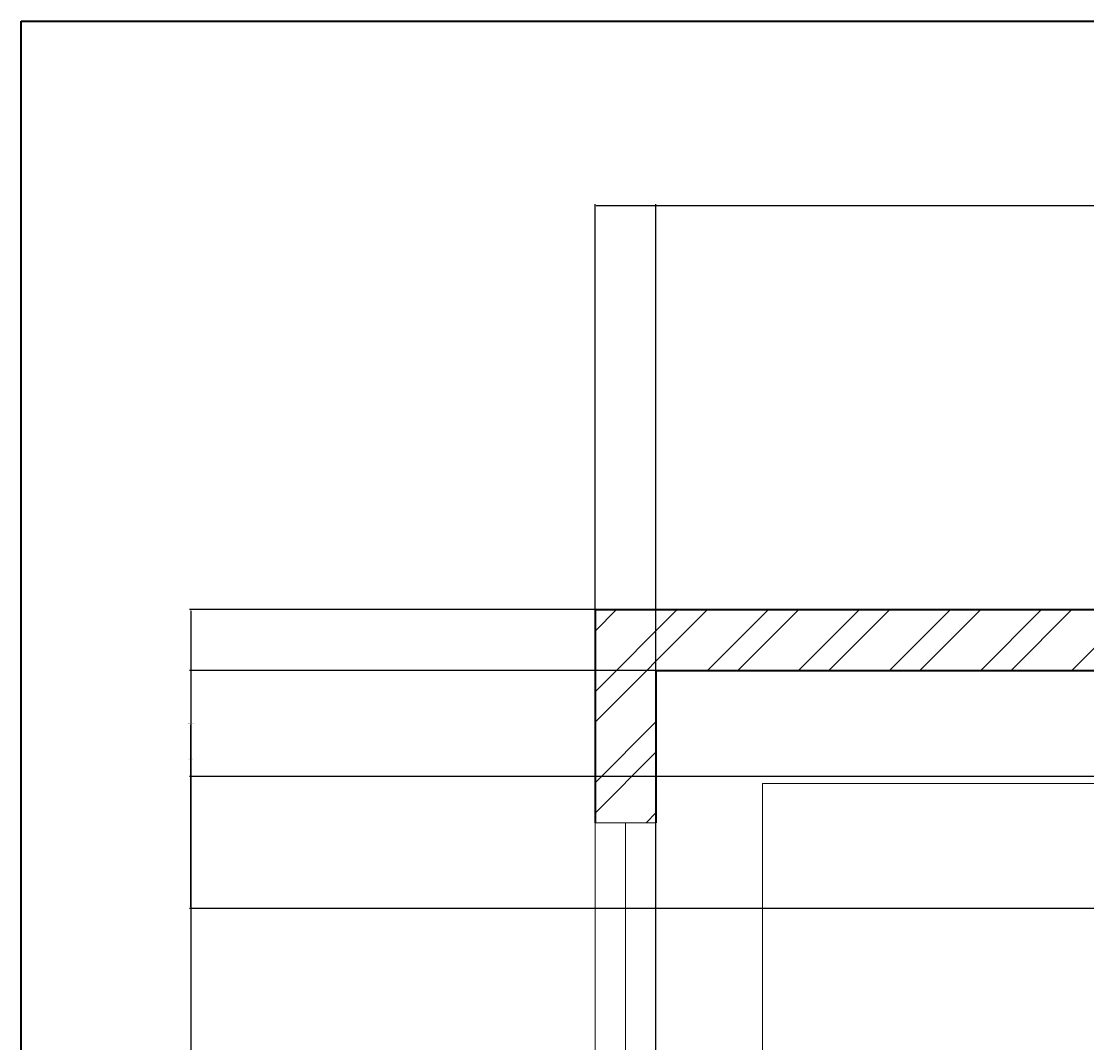
# Model space of a CAD drawing. Units: inches. Extents: x 2552 to 3217, y 1417 to 2737.
# Tile 17 of 25: x 2552 to 2710, y 2585 to 2737. Entities that reach past the tile are written whole.
import ezdxf

# ---------------------------------------------------------------- set-up
doc = ezdxf.new("R2010")
doc.units = ezdxf.units.IN
for name, color, linetype, lineweight in [('A-ANNO-DIMS', 2, 'Continuous', 18), ('A-ANNO-TTLB', 7, 'Continuous', 35), ('A-FLOR-CASE', 9, 'Continuous', 18), ('A-GLAZ', 161, 'Continuous', 18), ('A-WALL', 7, 'Continuous', 35), ('A-WALL-PATT', 217, 'Continuous', 13)]:
    doc.layers.add(name, color=color, linetype=linetype, lineweight=lineweight)
doc.styles.get("Standard").update_dxf_attribs({"font": 'arial.ttf'})
doc.dimstyles.get("Standard").update_dxf_attribs({"dimtxt": 0.18, "dimasz": 0.18, "dimexe": 0.18, "dimexo": 0.0625, "dimgap": 0.09, "dimtad": 0, "dimtih": 1, "dimtoh": 1, "dimdec": 4, "dimzin": 0, "dimdsep": 46, "dimtxsty": 'Standard', "dimcen": 0.09, "dimadec": 0, "dimazin": 0, "dimtfac": 1, "dimtdec": 4, "dimtofl": 0, "dimtmove": 0, "dimatfit": 3, "dimfxl": 1, "dimtolj": 1, "dimtzin": 0, "dimarcsym": 0})

# ---------------------------------------------------------------- blocks, each defined once
blk = doc.blocks.new('WIN-36')
for p, q in [((4.5, 36), (0, 36)), ((0, 36), (9, 36)), ((0, 36), (0, 0)), ((4.5, 0), (4.5, 36)), ((9, 36), (9, 0)), ((0, 0), (9, 0)), ((9, 0), (4.5, 0))]:
    blk.add_line(p, q)
blk = doc.blocks.new('*D50')
at = {"layer": 'A-ANNO-DIMS', "color": 0, "lineweight": -2, "transparency": 16777216}
for p, q in [((2637.29, 2649.51), (2577.37, 2649.51)), ((2577.55, 2649.33), (2577.55, 2096.19)), ((2577.55, 1542.69), (2577.55, 2095.83)), ((2637.29, 1542.51), (2577.37, 1542.51))]:
    blk.add_line(p, q, dxfattribs=at)
at = {"layer": 'A-ANNO-DIMS', "color": 0, "transparency": 16777216}
for points in [[(2577.52, 2649.33), (2577.58, 2649.33), (2577.55, 2649.51)], [(2577.52, 1542.69), (2577.58, 1542.69), (2577.55, 1542.51)]]:
    blk.add_solid(points, dxfattribs=at)
at = {"layer": 'Defpoints', "color": 0, "transparency": 16777216}
for p in [(2577.55, 2649.51), (2637.35, 2649.51), (2637.35, 1542.51)]:
    blk.add_point(p, dxfattribs=at)
at = {"layer": 'A-ANNO-DIMS', "color": 0, "transparency": 16777216, "insert": (2577.55, 2096.01), "char_height": 0.18, "attachment_point": 5}
blk.add_mtext('\\A1;1107', dxfattribs=at)
blk = doc.blocks.new('*D51')
at = {"layer": 'A-ANNO-DIMS', "color": 0, "lineweight": -2, "transparency": 16777216}
for p, q in [((2637.35, 2649.58), (2637.35, 2709.49)), ((2637.53, 2709.31), (2742.71, 2709.31)), ((2848.67, 2709.31), (2743.5, 2709.31)), ((2848.85, 2649.58), (2848.85, 2709.49))]:
    blk.add_line(p, q, dxfattribs=at)
at = {"layer": 'A-ANNO-DIMS', "color": 0, "transparency": 16777216}
for points in [[(2637.53, 2709.34), (2637.53, 2709.28), (2637.35, 2709.31)], [(2848.67, 2709.34), (2848.67, 2709.28), (2848.85, 2709.31)]]:
    blk.add_solid(points, dxfattribs=at)
at = {"layer": 'Defpoints', "color": 0, "transparency": 16777216}
for p in [(2848.85, 2709.31), (2637.35, 2649.51), (2848.85, 2649.51)]:
    blk.add_point(p, dxfattribs=at)
at = {"layer": 'A-ANNO-DIMS', "color": 0, "transparency": 16777216, "insert": (2743.1, 2709.31), "char_height": 0.18, "attachment_point": 5}
blk.add_mtext('\\A1;211.5', dxfattribs=at)
blk = doc.blocks.new('*D64')
at = {"layer": 'A-ANNO-DIMS', "color": 0, "lineweight": -2, "transparency": 16777216}
for p, q in [((2646.35, 1551.58), (2646.35, 2709.49)), ((2646.53, 2709.31), (2802.77, 2709.31)), ((2959.93, 2709.31), (2803.69, 2709.31)), ((2960.11, 1551.58), (2960.11, 2709.49))]:
    blk.add_line(p, q, dxfattribs=at)
at = {"layer": 'A-ANNO-DIMS', "color": 0, "transparency": 16777216}
for points in [[(2646.53, 2709.34), (2646.53, 2709.28), (2646.35, 2709.31)], [(2959.93, 2709.34), (2959.93, 2709.28), (2960.11, 2709.31)]]:
    blk.add_solid(points, dxfattribs=at)
at = {"layer": 'Defpoints', "color": 0, "transparency": 16777216}
for p in [(2960.11, 2709.31), (2646.35, 1551.51), (2960.11, 1551.51)]:
    blk.add_point(p, dxfattribs=at)
at = {"layer": 'A-ANNO-DIMS', "color": 0, "transparency": 16777216, "insert": (2803.23, 2709.31), "char_height": 0.18, "attachment_point": 5}
blk.add_mtext('\\A1;313.76', dxfattribs=at)
blk = doc.blocks.new('*D65')
at = {"layer": 'A-ANNO-DIMS', "color": 0, "lineweight": -2, "transparency": 16777216}
for p, q in [((2908.79, 2649.51), (2577.37, 2649.51)), ((2577.55, 2649.33), (2577.55, 2627.57)), ((2577.55, 2605.46), (2577.55, 2627.21)), ((2908.79, 2605.28), (2577.37, 2605.28))]:
    blk.add_line(p, q, dxfattribs=at)
at = {"layer": 'A-ANNO-DIMS', "color": 0, "transparency": 16777216}
for points in [[(2577.52, 2649.33), (2577.58, 2649.33), (2577.55, 2649.51)], [(2577.52, 2605.46), (2577.58, 2605.46), (2577.55, 2605.28)]]:
    blk.add_solid(points, dxfattribs=at)
at = {"layer": 'Defpoints', "color": 0, "transparency": 16777216}
for p in [(2577.55, 2649.51), (2908.85, 2649.51), (2908.85, 2605.28)]:
    blk.add_point(p, dxfattribs=at)
at = {"layer": 'A-ANNO-DIMS', "color": 0, "transparency": 16777216, "insert": (2577.55, 2627.39), "char_height": 0.18, "attachment_point": 5}
blk.add_mtext('\\A1;44.24', dxfattribs=at)
blk = doc.blocks.new('*D68')
at = {"layer": 'A-ANNO-DIMS', "color": 0, "lineweight": -2, "transparency": 16777216}
for p, q in [((2995.79, 2640.51), (2577.37, 2640.51)), ((2577.55, 2640.33), (2577.55, 2632.84)), ((2577.55, 2624.97), (2577.55, 2632.47)), ((2995.79, 2624.79), (2577.37, 2624.79))]:
    blk.add_line(p, q, dxfattribs=at)
at = {"layer": 'A-ANNO-DIMS', "color": 0, "transparency": 16777216}
for points in [[(2577.52, 2640.33), (2577.58, 2640.33), (2577.55, 2640.51)], [(2577.52, 2624.97), (2577.58, 2624.97), (2577.55, 2624.79)]]:
    blk.add_solid(points, dxfattribs=at)
at = {"layer": 'Defpoints', "color": 0, "transparency": 16777216}
for p in [(2995.85, 2640.51), (2577.55, 2624.79), (2995.85, 2624.79)]:
    blk.add_point(p, dxfattribs=at)
at = {"layer": 'A-ANNO-DIMS', "color": 0, "transparency": 16777216, "insert": (2577.55, 2632.65), "char_height": 0.18, "attachment_point": 5}
blk.add_mtext('\\A1;15.718', dxfattribs=at)

msp = doc.modelspace()

# ---------------------------------------------------------------- hatches: boundary and pattern name
at = {"layer": 'A-WALL-PATT'}
h = msp.add_hatch(dxfattribs=at)
h.set_pattern_fill('ANSI32', color=256)
h.paths.add_polyline_path([(2756.676, 2649.5125), (2637.3535, 2649.5125), (2637.3535, 2617.9626), (2641.8535, 2617.9626), (2646.3535, 2617.9626), (2646.3535, 2640.5125), (2724.3535, 2640.5125), (2724.3535, 2520.5125), (2720.299, 2520.5125), (2720.299, 2516.0125), (2733.4075, 2516.0125), (2733.4075, 2518.2213), (2733.4075, 2520.5125), (2728.8535, 2520.5125), (2728.8535, 2640.5125), (2756.676, 2640.5125)])
h.paths.add_polyline_path([(2848.8535, 2649.5125), (2804.676, 2649.5125), (2804.676, 2640.5125), (2839.8535, 2640.5125), (2839.8535, 2598.3517), (2848.8535, 2598.3517)])
h.paths.add_polyline_path([(2646.3535, 2516.0125), (2697.9593, 2516.0125), (2697.9593, 2518.2625), (2697.9593, 2520.5125), (2646.3535, 2520.5125), (2646.3535, 2581.9626), (2637.3535, 2581.9626), (2637.3535, 2364.3298), (2646.3535, 2364.3298), (2646.3535, 2387.0125), (2724.3535, 2387.0125), (2724.3535, 2267.0125), (2721.0443, 2267.0125), (2721.0443, 2262.5125), (2733.7854, 2262.5125), (2733.7854, 2264.7625), (2733.7854, 2267.0125), (2728.8535, 2267.0125), (2728.8535, 2387.0125), (2839.8535, 2387.0125), (2839.8535, 2363.8387), (2848.8535, 2363.8387), (2848.8535, 2403.7415), (2844.3535, 2403.7415), (2839.8535, 2403.7415), (2839.8535, 2396.0125), (2646.3535, 2396.0125)])
h.paths.add_polyline_path([(2848.8535, 2550.3517), (2844.3535, 2550.3517), (2839.8535, 2550.3517), (2839.8535, 2520.5125), (2801.9195, 2520.5125), (2801.9195, 2518.2625), (2801.9195, 2516.0125), (2839.8535, 2516.0125), (2839.8535, 2507.5813), (2848.8535, 2507.5813)], flags=17)
h.paths.add_polyline_path([(2848.8535, 2483.5813), (2844.3535, 2483.5813), (2839.8535, 2483.5813), (2839.8535, 2468.0125), (2773.8535, 2468.0125), (2773.8535, 2516.0125), (2778.1336, 2516.0125), (2778.1336, 2520.5125), (2766.696, 2520.5125), (2766.696, 2518.2625), (2766.696, 2516.0125), (2769.3535, 2516.0125), (2769.3535, 2463.5125), (2839.8535, 2463.5125), (2839.8535, 2431.0782), (2848.8535, 2431.0782)], flags=17)
h.paths.add_polyline_path([(2917.8535, 2569.2764), (2913.3535, 2569.2764), (2908.8535, 2569.2764), (2908.8535, 2433.001), (2917.8535, 2433.001), (2917.8535, 2516.0125), (2967.486, 2516.0125), (2967.486, 2520.5125), (2917.8535, 2520.5125)])
h.paths.add_polyline_path([(3000.3535, 2640.5125), (2995.8535, 2640.5125), (2995.8535, 2520.5125), (2990.688, 2520.5125), (2990.688, 2516.0125), (3004.0844, 2516.0125), (3004.0844, 2518.2625), (3004.0844, 2520.5125), (3000.3535, 2520.5125)])
h.paths.add_polyline_path([(3120.3535, 2561.3689), (3115.8535, 2561.3689), (3111.3535, 2561.3689), (3111.3535, 2520.5125), (3070.9814, 2520.5125), (3070.9814, 2518.2625), (3070.9814, 2516.0125), (3111.3535, 2516.0125), (3111.3535, 2505.1841), (3120.3535, 2505.1841)])
h.paths.add_polyline_path([(3120.3535, 2481.1841), (3115.8535, 2481.1841), (3111.3535, 2481.1841), (3111.3535, 2468.0125), (3045.3535, 2468.0125), (3045.3535, 2516.0125), (3048.9787, 2516.0125), (3048.9787, 2520.5125), (3036.3395, 2520.5125), (3036.3395, 2516.0125), (3040.8535, 2516.0125), (3040.8535, 2463.5125), (3111.3535, 2463.5125), (3111.3535, 2396.0125), (2917.8535, 2396.0125), (2917.8535, 2403.4124), (2913.3535, 2403.4124), (2908.8535, 2403.4124), (2908.8535, 2182.5756), (2917.8535, 2182.5756), (2917.8535, 2262.5125), (2968.001, 2262.5125), (2968.001, 2264.7625), (2968.001, 2267.0125), (2917.8535, 2267.0125), (2917.8535, 2387.0125), (3111.3535, 2387.0125), (3111.3535, 2352.2435), (3120.3535, 2352.2435)])
h.paths.add_polyline_path([(3120.3535, 2304.2435), (3115.8535, 2304.2435), (3111.3535, 2304.2435), (3111.3535, 2267.0125), (3073.8616, 2267.0125), (3073.8616, 2264.7625), (3073.8616, 2262.5125), (3111.3535, 2262.5125), (3111.3535, 2252.376), (3120.3535, 2252.376)], flags=17)
h.paths.add_polyline_path([(3120.3535, 2228.376), (3115.8535, 2228.376), (3111.3535, 2228.376), (3111.3535, 2214.5125), (3045.3535, 2214.5125), (3045.3535, 2262.5125), (3049.3096, 2262.5125), (3049.3096, 2267.0125), (3035.0125, 2267.0125), (3035.0125, 2262.5125), (3040.8535, 2262.5125), (3040.8535, 2210.0125), (3111.3535, 2210.0125), (3111.3535, 2142.5125), (2917.8535, 2142.5125), (2917.8535, 2150.2408), (2913.3535, 2150.2408), (2908.8535, 2150.2408), (2908.8535, 1924.9905), (2917.8535, 1924.9905), (2917.8535, 2009.0125), (2971.959, 2009.0125), (2971.959, 2011.2625), (2971.959, 2013.5125), (2917.8535, 2013.5125), (2917.8535, 2133.5125), (2995.8535, 2133.5125), (2995.8535, 2013.5125), (2992.1797, 2013.5125), (2992.1797, 2009.0125), (3004.3344, 2009.0125), (3004.3344, 2011.2625), (3004.3344, 2013.5125), (3000.3535, 2013.5125), (3000.3535, 2133.5125), (3111.3535, 2133.5125), (3111.3535, 2115.0291), (3120.3535, 2115.0291)])
h.paths.add_polyline_path([(3000.3535, 2387.0125), (2995.8535, 2387.0125), (2995.8535, 2267.0125), (2991.3326, 2267.0125), (2991.3326, 2262.5125), (3004.1044, 2262.5125), (3004.1044, 2264.7625), (3004.1044, 2267.0125), (3000.3535, 2267.0125)], flags=17)
h.paths.add_polyline_path([(3120.3535, 1973.2388), (3115.8535, 1973.2388), (3111.3535, 1973.2388), (3111.3535, 1961.0125), (3045.3535, 1961.0125), (3045.3535, 2009.0125), (3048.9101, 2009.0125), (3048.9101, 2013.5125), (3037.105, 2013.5125), (3037.105, 2011.2625), (3037.105, 2009.0125), (3040.8535, 2009.0125), (3040.8535, 1956.5125), (3111.3535, 1956.5125), (3111.3535, 1889.0125), (2917.8535, 1889.0125), (2917.8535, 1895.7215), (2913.3535, 1895.7215), (2908.8535, 1895.7215), (2908.8535, 1844.2217), (2917.8535, 1844.2217), (2917.8535, 1880.0125), (3111.3535, 1880.0125), (3111.3535, 1846.9541), (3120.3535, 1846.9541)])
h.paths.add_polyline_path([(3120.3535, 2067.0291), (3111.3535, 2067.0291), (3111.3535, 2013.5125), (3071.3001, 2013.5125), (3071.3001, 2009.0125), (3111.3535, 2009.0125), (3111.3535, 1997.2388), (3120.3535, 1997.2388)], flags=0)
h.paths.add_polyline_path([(3120.3535, 1798.9541), (3115.8535, 1798.9541), (3111.3535, 1798.9541), (3111.3535, 1760.0125), (3071.2497, 1760.0125), (3071.2497, 1757.7625), (3071.2497, 1755.5125), (3111.3535, 1755.5125), (3111.3535, 1746.162), (3120.3535, 1746.2478)])
h.paths.add_polyline_path([(3120.3535, 1722.2049), (3111.3535, 1722.2049), (3111.3535, 1707.5125), (3045.3535, 1707.5125), (3045.3535, 1755.5125), (3048.6624, 1755.5125), (3048.6624, 1760.0125), (3035.3703, 1760.0125), (3035.3703, 1755.5125), (3040.8535, 1755.5125), (3040.8535, 1703.0125), (3111.3535, 1703.0125), (3111.3535, 1635.5125), (2917.8535, 1635.5125), (2917.8535, 1643.1366), (2913.3535, 1643.1366), (2908.8535, 1643.1366), (2908.8535, 1626.5125), (3120.3535, 1626.5125)])
h.paths.add_polyline_path([(2917.8535, 1755.5125), (2973.2287, 1755.5125), (2973.2287, 1757.7625), (2973.2287, 1760.0125), (2917.8535, 1760.0125), (2917.8535, 1808.2217), (2913.3535, 1808.2217), (2908.8535, 1808.2217), (2908.8535, 1676.1665), (2917.8535, 1676.1665)])
h.paths.add_polyline_path([(3000.3535, 1880.0125), (2995.8535, 1880.0125), (2995.8535, 1760.0125), (2992.9329, 1760.0125), (2992.9329, 1755.5125), (3003.8766, 1755.5125), (3003.8766, 1757.7625), (3003.8766, 1760.0125), (3000.3535, 1760.0125)])
h.paths.add_polyline_path([(2848.8535, 1896.6971), (2844.3535, 1896.6971), (2839.8535, 1896.6971), (2839.8535, 1889.0125), (2646.3535, 1889.0125), (2646.3535, 2009.0125), (2700.5253, 2009.0125), (2700.5253, 2011.2625), (2700.5253, 2013.5125), (2646.3535, 2013.5125), (2646.3535, 2053.1812), (2641.8535, 2053.1812), (2637.3535, 2053.1812), (2637.3535, 1836.254), (2646.3535, 1836.254), (2646.3535, 1880.0125), (2724.3535, 1880.0125), (2724.3535, 1760.0125), (2721.2473, 1760.0125), (2721.2473, 1755.5125), (2731.9187, 1755.5125), (2731.9187, 1757.7625), (2731.9187, 1760.0125), (2728.8535, 1760.0125), (2728.8535, 1880.0125), (2839.8535, 1880.0125), (2839.8535, 1840.3813), (2848.8535, 1840.3813)])
h.paths.add_polyline_path([(2848.8535, 1792.3813), (2844.3535, 1792.3813), (2839.8535, 1792.3813), (2839.8535, 1760.0125), (2797.8845, 1760.0125), (2797.8845, 1755.5125), (2839.8535, 1755.5125), (2839.8535, 1743.3688), (2844.3535, 1743.3688), (2848.8535, 1743.3688)], flags=0)
h.paths.add_polyline_path([(2848.8535, 1719.3688), (2844.3535, 1719.3688), (2839.8535, 1719.3688), (2839.8535, 1707.5125), (2773.8535, 1707.5125), (2773.8535, 1755.5125), (2777.716, 1755.5125), (2777.716, 1760.0125), (2760.9247, 1760.0125), (2760.9247, 1757.9721), (2760.9247, 1755.5125), (2769.3535, 1755.5125), (2769.3535, 1703.0125), (2839.8535, 1703.0125), (2839.8535, 1673.0277), (2848.8535, 1672.9407)], flags=0)
h.paths.add_polyline_path([(2646.3535, 1755.5125), (2702.9171, 1755.5125), (2702.9171, 1757.7625), (2702.9171, 1760.0125), (2646.3535, 1760.0125), (2646.3535, 1800.254), (2641.8535, 1800.254), (2637.3535, 1800.254), (2637.3535, 1626.5125), (2848.8535, 1626.5125), (2848.8535, 1643.1187), (2844.3535, 1643.1187), (2839.8535, 1643.1187), (2839.8535, 1635.5125), (2646.3535, 1635.5125)])
h.paths.add_polyline_path([(2848.8535, 2148.8427), (2844.3535, 2148.8427), (2839.8535, 2148.8427), (2839.8535, 2142.5125), (2646.3535, 2142.5125), (2646.3535, 2262.5125), (2701.3562, 2262.5125), (2701.3562, 2264.7625), (2701.3562, 2267.0125), (2646.3535, 2267.0125), (2646.3535, 2328.3298), (2637.3535, 2328.3298), (2637.3535, 2089.1812), (2646.3535, 2089.1812), (2646.3535, 2133.5125), (2839.8535, 2133.5125), (2839.8535, 2097.5966), (2848.8535, 2097.5966)])
h.paths.add_polyline_path([(2728.8535, 2133.5125), (2724.3535, 2133.5125), (2724.3535, 2013.5125), (2719.6039, 2013.5125), (2719.6039, 2009.0125), (2732.5784, 2009.0125), (2732.5784, 2011.2625), (2732.5784, 2013.5125), (2728.8535, 2013.5125)])
h.paths.add_polyline_path([(2848.8535, 1970.0557), (2844.3535, 1970.0557), (2839.8535, 1970.0557), (2839.8535, 1961.0125), (2773.8535, 1961.0125), (2773.8535, 2009.0125), (2777.3388, 2009.0125), (2777.3388, 2013.5125), (2764.7681, 2013.5125), (2764.7681, 2009.0125), (2769.3535, 2009.0125), (2769.3535, 1956.5125), (2839.8535, 1956.5125), (2839.8535, 1924.7199), (2848.8535, 1924.7199)], flags=17)
h.paths.add_polyline_path([(2848.8535, 2049.5966), (2844.3535, 2049.5966), (2839.8535, 2049.5966), (2839.8535, 2013.5125), (2798.198, 2013.5125), (2798.198, 2011.2625), (2798.198, 2009.0125), (2839.8535, 2009.0125), (2839.8535, 1994.0557), (2848.8535, 1994.0557)], flags=17)
h.paths.add_polyline_path([(2848.8535, 2315.8387), (2839.8535, 2315.8387), (2839.8535, 2267.0125), (2799.3375, 2267.0125), (2799.3375, 2264.7625), (2799.3375, 2262.5125), (2839.8535, 2262.5125), (2839.8535, 2253.2843), (2848.8535, 2253.2843)], flags=17)
h.paths.add_polyline_path([(2848.8535, 2229.2843), (2839.8535, 2229.2843), (2839.8535, 2177.6936), (2848.8535, 2177.6936)], flags=17)
h.paths.add_polyline_path([(2839.8535, 2214.5125), (2773.8535, 2214.5125), (2773.8535, 2262.5125), (2777.6984, 2262.5125), (2777.6984, 2267.0125), (2763.8226, 2267.0125), (2763.8226, 2262.5125), (2769.3535, 2262.5125), (2769.3535, 2210.0125), (2839.8535, 2210.0125)], flags=17)
h.paths.add_polyline_path([(3050.32, 2520.2817), (3088.9114, 2520.2817), (3088.9114, 2538.939), (3050.32, 2538.939)], flags=9)

# ---------------------------------------------------------------- linework, layer by layer
at = {"layer": 'A-ANNO-TTLB'}
msp.add_lwpolyline([(2552.473, 2736.5692), (3216.7862, 2736.5692), (3216.7862, 1416.6914), (2552.473, 1416.6914)], close=True, dxfattribs=at)
at = {"layer": 'A-FLOR-CASE'}
for p, q in [((2662.102, 2520.5125), (2662.102, 2623.7542)), ((2662.102, 2623.7542), (2724.3535, 2623.7542))]:
    msp.add_line(p, q, dxfattribs=at)
at = {"layer": 'A-WALL'}
for p, q in [((2637.3535, 2649.5125), (2756.676, 2649.5125)), ((2637.3535, 2649.5125), (2637.3535, 2617.9626)), ((2646.3535, 2640.5125), (2724.3535, 2640.5125)), ((2646.3535, 2640.5125), (2646.3535, 2617.9626))]:
    msp.add_line(p, q, dxfattribs=at)

# ---------------------------------------------------------------- block references
at = {"layer": 'A-GLAZ'}
msp.add_blockref('WIN-36', (2637.354, 2581.9629), dxfattribs=at)

# ---------------------------------------------------------------- dimensions: what is measured, and where the dimension line sits
at = {"layer": 'A-ANNO-DIMS'}
for base, p1, p2, override, picture, middle in [((2848.8535, 2709.3125), (2637.3535, 2649.5125), (2848.8535, 2649.5125), {"dimdec": 1, "dimlfac": 1, "dimrnd": 0, "dimzin": 0, "dimdsep": 46, "dimlunit": 2}, '*D51', (2743.1035, 2709.3125)), ((2960.1089, 2709.3125), (2646.3535, 1551.5125), (2960.1089, 1551.5125), {"dimdec": 2, "dimlfac": 1, "dimrnd": 0, "dimzin": 0, "dimdsep": 46, "dimlunit": 2}, '*D64', (2803.2312, 2709.3125))]:
    dim = msp.add_linear_dim(base=base, p1=p1, p2=p2, dimstyle='Standard', override=override, dxfattribs=at)
    dim.commit()
    dim.dimension.update_dxf_attribs({"geometry": picture, "text_midpoint": middle})
for base, p1, p2, override, picture, middle in [((2577.5535, 2649.5125), (2908.8535, 2605.2764), (2908.8535, 2649.5125), {"dimdec": 2, "dimlfac": 1, "dimrnd": 0, "dimzin": 0, "dimdsep": 46, "dimlunit": 2}, '*D65', (2577.5535, 2627.3945)), ((2577.5535, 2649.5125), (2637.3535, 1542.5125), (2637.3535, 2649.5125), {"dimdec": 0, "dimlfac": 1, "dimrnd": 0, "dimzin": 0, "dimdsep": 46, "dimlunit": 2}, '*D50', (2577.5535, 2096.0125)), ((2577.5535, 2624.7942), (2995.8535, 2640.5125), (2995.8535, 2624.7942), {"dimdec": 3, "dimlfac": 1, "dimrnd": 0, "dimzin": 0, "dimdsep": 46, "dimlunit": 2}, '*D68', (2577.5535, 2632.6534))]:
    dim = msp.add_linear_dim(base=base, p1=p1, p2=p2, angle=90, dimstyle='Standard', override=override, dxfattribs=at)
    dim.commit()
    dim.dimension.update_dxf_attribs({"geometry": picture, "text_midpoint": middle})

doc.saveas('drawing.dxf')
